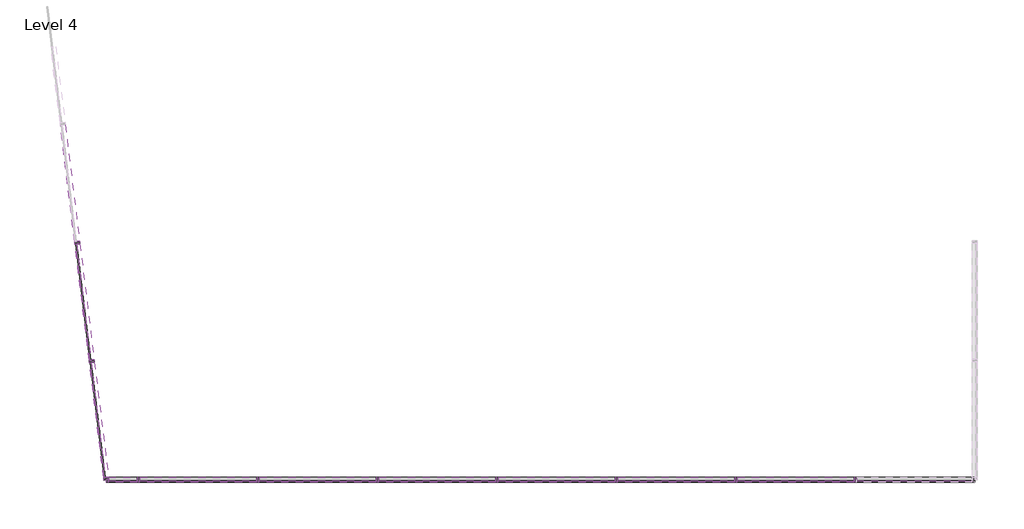
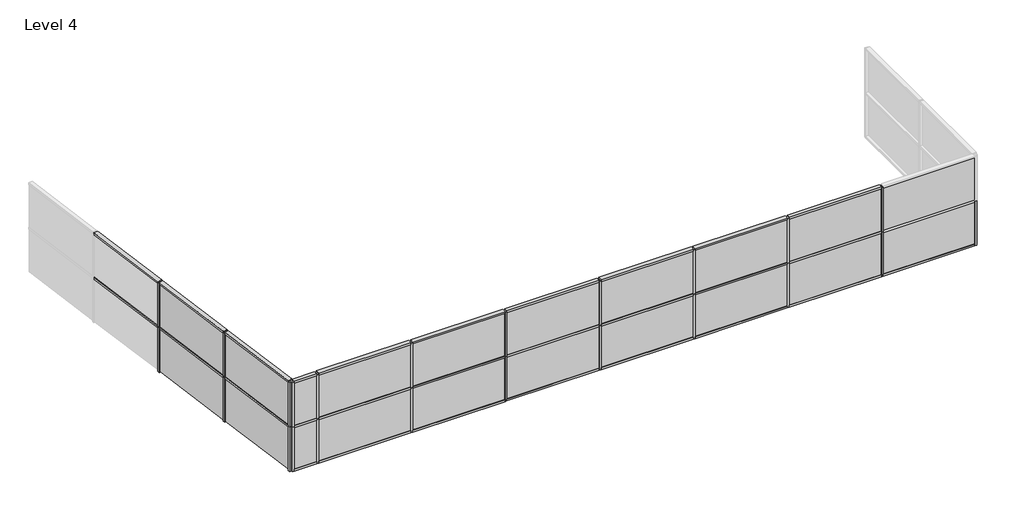
# One storey, part 1 of 2: 51 members, 20 plates.
"""IFC4 building model written with IfcOpenShell, lengths in millimetres."""

from ifc_helpers import new_model, si_unit, origin, place, context, project, spatial, transform, mapped, element, save
from components import member_71c27fd2, member_19d0a4ec, member_8cef0660, member_db480205, member_82905deb, member_4491d118, member_695b83e4, member_0c11e56c, system_panel_glazed_37f15d2e, system_panel_glazed_3620f98e, system_panel_glazed_e46d4b42, system_panel_glazed_2a6c68b7, system_panel_glazed_07b088f8, system_panel_glazed_9d0e0944

model = new_model("IFC4")

# Units and contexts
model_context = context("Model", 3, world=origin())
ifc_project = project(units=[si_unit("LENGTHUNIT", "METRE", prefix="MILLI")], contexts=[model_context])

# Site, building, storey
site = spatial("IfcSite", under=ifc_project)
building = spatial("IfcBuilding", under=site)
storey = spatial("IfcBuildingStorey", under=building, Name="Level 4", Elevation=9144.0)

# Members
placement = place(None, origin())
member_shape = member_71c27fd2(model_context)
element("IfcMember", 1, ObjectType="Rectangular Mullion : 2.5\" x 5\" rectangular", at=placement, inside=storey, context=model_context, shape_type="MappedRepresentation", body=[
    mapped(member_shape, transform((10886.265636, -6979.1363705, 9144.0), x_axis=(0.0, 0.0, -1.0), y_axis=(0.0, -1.0, 0.0), z_axis=(-1.0, 0.0, 0.0))),
])
member_2_shape = member_19d0a4ec(model_context)
element("IfcMember", 2, ObjectType="Rectangular Mullion : 2.5\" x 5\" rectangular", at=placement, inside=storey, context=model_context, shape_type="MappedRepresentation", body=[
    mapped(member_2_shape, transform((-8260.4765148, -6916.1096898, 10668.0), x_axis=(0.0, 0.0, 1.0), y_axis=(-0.9925461516413222, -0.12186934340514594, 0.0), z_axis=(0.12186934340514592, -0.9925461516413221, 0.0))),
])
element("IfcMember", 3, ObjectType="Rectangular Mullion : 2.5\" x 5\" rectangular", at=placement, inside=storey, context=model_context, shape_type="MappedRepresentation", body=[
    mapped(member_2_shape, transform((-8260.4765148, -6916.1096898, 12192.0), x_axis=(0.0, 0.0, 1.0), y_axis=(-0.9925461516413222, -0.1218693434051461, 0.0), z_axis=(0.1218693434051461, -0.9925461516413222, 0.0))),
])
member_3_shape = member_8cef0660(model_context)
element("IfcMember", 4, ObjectType="Rectangular Mullion : 2.5\" x 5\" rectangular", at=placement, inside=storey, context=model_context, shape_type="MappedRepresentation", body=[
    mapped(member_3_shape, transform((10822.765636, -6979.1363705, 10668.0), x_axis=(0.0, 0.0, 1.0), y_axis=(0.0, -1.0, 0.0), z_axis=(1.0, 0.0, 0.0))),
])
element("IfcMember", 5, ObjectType="Rectangular Mullion : 2.5\" x 5\" rectangular", at=placement, inside=storey, context=model_context, shape_type="MappedRepresentation", body=[
    mapped(member_3_shape, transform((7774.765636, -6979.1363705, 10668.0), x_axis=(0.0, 0.0, 1.0), y_axis=(0.0, -1.0, 0.0), z_axis=(1.0, 0.0, 0.0))),
])
element("IfcMember", 6, ObjectType="Rectangular Mullion : 2.5\" x 5\" rectangular", at=placement, inside=storey, context=model_context, shape_type="MappedRepresentation", body=[
    mapped(member_3_shape, transform((4726.765636, -6979.1363705, 10668.0), x_axis=(0.0, 0.0, 1.0), y_axis=(0.0, -1.0, 0.0), z_axis=(1.0, 0.0, 0.0))),
])
element("IfcMember", 7, ObjectType="Rectangular Mullion : 2.5\" x 5\" rectangular", at=placement, inside=storey, context=model_context, shape_type="MappedRepresentation", body=[
    mapped(member_3_shape, transform((1678.765636, -6979.1363705, 10668.0), x_axis=(0.0, 0.0, 1.0), y_axis=(0.0, -1.0, 0.0), z_axis=(1.0, 0.0, 0.0))),
])
element("IfcMember", 8, ObjectType="Rectangular Mullion : 2.5\" x 5\" rectangular", at=placement, inside=storey, context=model_context, shape_type="MappedRepresentation", body=[
    mapped(member_3_shape, transform((-1369.234364, -6979.1363705, 10668.0), x_axis=(0.0, 0.0, 1.0), y_axis=(0.0, -1.0, 0.0), z_axis=(1.0, 0.0, 0.0))),
])
element("IfcMember", 9, ObjectType="Rectangular Mullion : 2.5\" x 5\" rectangular", at=placement, inside=storey, context=model_context, shape_type="MappedRepresentation", body=[
    mapped(member_3_shape, transform((-4417.234364, -6979.1363705, 10668.0), x_axis=(0.0, 0.0, 1.0), y_axis=(0.0, -1.0, 0.0), z_axis=(1.0, 0.0, 0.0))),
])
element("IfcMember", 10, ObjectType="Rectangular Mullion : 2.5\" x 5\" rectangular", at=placement, inside=storey, context=model_context, shape_type="MappedRepresentation", body=[
    mapped(member_3_shape, transform((10822.765636, -6979.1363705, 12192.0), x_axis=(0.0, 0.0, 1.0), y_axis=(0.0, -1.0, 0.0), z_axis=(1.0, 0.0, 0.0))),
])
element("IfcMember", 11, ObjectType="Rectangular Mullion : 2.5\" x 5\" rectangular", at=placement, inside=storey, context=model_context, shape_type="MappedRepresentation", body=[
    mapped(member_3_shape, transform((7774.765636, -6979.1363705, 12192.0), x_axis=(0.0, 0.0, 1.0), y_axis=(0.0, -1.0, 0.0), z_axis=(1.0, 0.0, 0.0))),
])
element("IfcMember", 12, ObjectType="Rectangular Mullion : 2.5\" x 5\" rectangular", at=placement, inside=storey, context=model_context, shape_type="MappedRepresentation", body=[
    mapped(member_3_shape, transform((4726.765636, -6979.1363705, 12192.0), x_axis=(0.0, 0.0, 1.0), y_axis=(0.0, -1.0, 0.0), z_axis=(1.0, 0.0, 0.0))),
])
element("IfcMember", 13, ObjectType="Rectangular Mullion : 2.5\" x 5\" rectangular", at=placement, inside=storey, context=model_context, shape_type="MappedRepresentation", body=[
    mapped(member_3_shape, transform((1678.765636, -6979.1363705, 12192.0), x_axis=(0.0, 0.0, 1.0), y_axis=(0.0, -1.0, 0.0), z_axis=(1.0, 0.0, 0.0))),
])
element("IfcMember", 14, ObjectType="Rectangular Mullion : 2.5\" x 5\" rectangular", at=placement, inside=storey, context=model_context, shape_type="MappedRepresentation", body=[
    mapped(member_3_shape, transform((-1369.234364, -6979.1363705, 12192.0), x_axis=(0.0, 0.0, 1.0), y_axis=(0.0, -1.0, 0.0), z_axis=(1.0, 0.0, 0.0))),
])
element("IfcMember", 15, ObjectType="Rectangular Mullion : 2.5\" x 5\" rectangular", at=placement, inside=storey, context=model_context, shape_type="MappedRepresentation", body=[
    mapped(member_3_shape, transform((-4417.234364, -6979.1363705, 12192.0), x_axis=(0.0, 0.0, 1.0), y_axis=(0.0, -1.0, 0.0), z_axis=(1.0, 0.0, 0.0))),
])
element("IfcMember", 16, ObjectType="Rectangular Mullion : 2.5\" x 5\" rectangular", at=placement, inside=storey, context=model_context, shape_type="MappedRepresentation", body=[
    mapped(member_3_shape, transform((-8628.0649219, -3922.3423596, 10668.0), x_axis=(0.0, 0.0, 1.0), y_axis=(-0.9925461516413222, -0.12186934340514595, 0.0), z_axis=(0.12186934340514595, -0.9925461516413222, 0.0))),
])
element("IfcMember", 17, ObjectType="Rectangular Mullion : 2.5\" x 5\" rectangular", at=placement, inside=storey, context=model_context, shape_type="MappedRepresentation", body=[
    mapped(member_3_shape, transform((-8999.5226806, -897.0616894, 10668.0), x_axis=(0.0, 0.0, 1.0), y_axis=(-0.9925461516413222, -0.12186934340514602, 0.0), z_axis=(0.12186934340514602, -0.9925461516413222, 0.0))),
])
element("IfcMember", 18, ObjectType="Rectangular Mullion : 2.5\" x 5\" rectangular", at=placement, inside=storey, context=model_context, shape_type="MappedRepresentation", body=[
    mapped(member_3_shape, transform((-8628.0649219, -3922.3423596, 12192.0), x_axis=(0.0, 0.0, 1.0), y_axis=(-0.9925461516413222, -0.12186934340514595, 0.0), z_axis=(0.12186934340514595, -0.9925461516413222, 0.0))),
])
element("IfcMember", 19, ObjectType="Rectangular Mullion : 2.5\" x 5\" rectangular", at=placement, inside=storey, context=model_context, shape_type="MappedRepresentation", body=[
    mapped(member_3_shape, transform((-8999.5226806, -897.0616894, 12192.0), x_axis=(0.0, 0.0, 1.0), y_axis=(-0.9925461516413222, -0.12186934340514566, 0.0), z_axis=(0.12186934340514566, -0.9925461516413222, 0.0))),
])
member_4_shape = member_db480205(model_context)
element("IfcMember", 20, ObjectType="Rectangular Mullion : 2.5\" x 5\" rectangular", at=placement, inside=storey, context=model_context, shape_type="MappedRepresentation", body=[
    mapped(member_4_shape, transform((7838.265636, -6979.1363705, 9144.0), x_axis=(0.0, 0.0, -1.0), y_axis=(0.0, -1.0, 0.0), z_axis=(-1.0, 0.0, 0.0))),
])
element("IfcMember", 21, ObjectType="Rectangular Mullion : 2.5\" x 5\" rectangular", at=placement, inside=storey, context=model_context, shape_type="MappedRepresentation", body=[
    mapped(member_4_shape, transform((4790.265636, -6979.1363705, 9144.0), x_axis=(0.0, 0.0, -1.0), y_axis=(0.0, -1.0, 0.0), z_axis=(-1.0, 0.0, 0.0))),
])
element("IfcMember", 22, ObjectType="Rectangular Mullion : 2.5\" x 5\" rectangular", at=placement, inside=storey, context=model_context, shape_type="MappedRepresentation", body=[
    mapped(member_4_shape, transform((1742.265636, -6979.1363705, 9144.0), x_axis=(0.0, 0.0, -1.0), y_axis=(0.0, -1.0, 0.0), z_axis=(-1.0, 0.0, 0.0))),
])
element("IfcMember", 23, ObjectType="Rectangular Mullion : 2.5\" x 5\" rectangular", at=placement, inside=storey, context=model_context, shape_type="MappedRepresentation", body=[
    mapped(member_4_shape, transform((-1305.734364, -6979.1363705, 9144.0), x_axis=(0.0, 0.0, -1.0), y_axis=(0.0, -1.0, 0.0), z_axis=(-1.0, 0.0, 0.0))),
])
element("IfcMember", 24, ObjectType="Rectangular Mullion : 2.5\" x 5\" rectangular", at=placement, inside=storey, context=model_context, shape_type="MappedRepresentation", body=[
    mapped(member_4_shape, transform((-4353.734364, -6979.1363705, 9144.0), x_axis=(0.0, 0.0, -1.0), y_axis=(0.0, -1.0, 0.0), z_axis=(-1.0, 0.0, 0.0))),
])
element("IfcMember", 25, ObjectType="Rectangular Mullion : 2.5\" x 5\" rectangular", at=placement, inside=storey, context=model_context, shape_type="MappedRepresentation", body=[
    mapped(member_4_shape, transform((-7401.734364, -6979.1363705, 9144.0), x_axis=(0.0, 0.0, -1.0), y_axis=(0.0, -1.0, 0.0), z_axis=(-1.0, 0.0, 0.0))),
])
member_5_shape = member_82905deb(model_context)
element("IfcMember", 26, ObjectType="Rectangular Mullion : 2.5\" x 5\" rectangular", at=placement, inside=storey, context=model_context, shape_type="MappedRepresentation", body=[
    mapped(member_5_shape, transform((10854.515636, -6979.1363705, 10668.0), x_axis=(-1.0, 0.0, 0.0), y_axis=(0.0, -1.0, 0.0), z_axis=(0.0, 0.0, 1.0))),
])
element("IfcMember", 27, ObjectType="Rectangular Mullion : 2.5\" x 5\" rectangular", at=placement, inside=storey, context=model_context, shape_type="MappedRepresentation", body=[
    mapped(member_5_shape, transform((7806.515636, -6979.1363705, 10668.0), x_axis=(-1.0, 0.0, 0.0), y_axis=(0.0, -1.0, 0.0), z_axis=(0.0, 0.0, 1.0))),
])
element("IfcMember", 28, ObjectType="Rectangular Mullion : 2.5\" x 5\" rectangular", at=placement, inside=storey, context=model_context, shape_type="MappedRepresentation", body=[
    mapped(member_5_shape, transform((4758.515636, -6979.1363705, 10668.0), x_axis=(-1.0, 0.0, 0.0), y_axis=(0.0, -1.0, 0.0), z_axis=(0.0, 0.0, 1.0))),
])
element("IfcMember", 29, ObjectType="Rectangular Mullion : 2.5\" x 5\" rectangular", at=placement, inside=storey, context=model_context, shape_type="MappedRepresentation", body=[
    mapped(member_5_shape, transform((1710.515636, -6979.1363705, 10668.0), x_axis=(-1.0, 0.0, 0.0), y_axis=(0.0, -1.0, 0.0), z_axis=(0.0, 0.0, 1.0))),
])
element("IfcMember", 30, ObjectType="Rectangular Mullion : 2.5\" x 5\" rectangular", at=placement, inside=storey, context=model_context, shape_type="MappedRepresentation", body=[
    mapped(member_5_shape, transform((-1337.484364, -6979.1363705, 10668.0), x_axis=(-1.0, 0.0, 0.0), y_axis=(0.0, -1.0, 0.0), z_axis=(0.0, 0.0, 1.0))),
])
element("IfcMember", 31, ObjectType="Rectangular Mullion : 2.5\" x 5\" rectangular", at=placement, inside=storey, context=model_context, shape_type="MappedRepresentation", body=[
    mapped(member_5_shape, transform((-4385.484364, -6979.1363705, 10668.0), x_axis=(-1.0, 0.0, 0.0), y_axis=(0.0, -1.0, 0.0), z_axis=(0.0, 0.0, 1.0))),
])
element("IfcMember", 32, ObjectType="Rectangular Mullion : 2.5\" x 5\" rectangular", at=placement, inside=storey, context=model_context, shape_type="MappedRepresentation", body=[
    mapped(member_5_shape, transform((-7433.484364, -6979.1363705, 10668.0), x_axis=(-1.0, 0.0, 0.0), y_axis=(0.0, -1.0, 0.0), z_axis=(0.0, 0.0, 1.0))),
])
element("IfcMember", 33, ObjectType="Rectangular Mullion : 2.5\" x 5\" rectangular", at=placement, inside=storey, context=model_context, shape_type="MappedRepresentation", body=[
    mapped(member_5_shape, transform((10854.515636, -6979.1363705, 12192.0), x_axis=(-1.0, 0.0, 0.0), y_axis=(0.0, -1.0, 0.0), z_axis=(0.0, 0.0, 1.0))),
])
element("IfcMember", 34, ObjectType="Rectangular Mullion : 2.5\" x 5\" rectangular", at=placement, inside=storey, context=model_context, shape_type="MappedRepresentation", body=[
    mapped(member_5_shape, transform((7806.515636, -6979.1363705, 12192.0), x_axis=(-1.0, 0.0, 0.0), y_axis=(0.0, -1.0, 0.0), z_axis=(0.0, 0.0, 1.0))),
])
element("IfcMember", 35, ObjectType="Rectangular Mullion : 2.5\" x 5\" rectangular", at=placement, inside=storey, context=model_context, shape_type="MappedRepresentation", body=[
    mapped(member_5_shape, transform((4758.515636, -6979.1363705, 12192.0), x_axis=(-1.0, 0.0, 0.0), y_axis=(0.0, -1.0, 0.0), z_axis=(0.0, 0.0, 1.0))),
])
element("IfcMember", 36, ObjectType="Rectangular Mullion : 2.5\" x 5\" rectangular", at=placement, inside=storey, context=model_context, shape_type="MappedRepresentation", body=[
    mapped(member_5_shape, transform((1710.515636, -6979.1363705, 12192.0), x_axis=(-1.0, 0.0, 0.0), y_axis=(0.0, -1.0, 0.0), z_axis=(0.0, 0.0, 1.0))),
])
element("IfcMember", 37, ObjectType="Rectangular Mullion : 2.5\" x 5\" rectangular", at=placement, inside=storey, context=model_context, shape_type="MappedRepresentation", body=[
    mapped(member_5_shape, transform((-1337.484364, -6979.1363705, 12192.0), x_axis=(-1.0, 0.0, 0.0), y_axis=(0.0, -1.0, 0.0), z_axis=(0.0, 0.0, 1.0))),
])
element("IfcMember", 38, ObjectType="Rectangular Mullion : 2.5\" x 5\" rectangular", at=placement, inside=storey, context=model_context, shape_type="MappedRepresentation", body=[
    mapped(member_5_shape, transform((-4385.484364, -6979.1363705, 12192.0), x_axis=(-1.0, 0.0, 0.0), y_axis=(0.0, -1.0, 0.0), z_axis=(0.0, 0.0, 1.0))),
])
element("IfcMember", 39, ObjectType="Rectangular Mullion : 2.5\" x 5\" rectangular", at=placement, inside=storey, context=model_context, shape_type="MappedRepresentation", body=[
    mapped(member_5_shape, transform((-7433.484364, -6979.1363705, 12192.0), x_axis=(-1.0, 0.0, 0.0), y_axis=(0.0, -1.0, 0.0), z_axis=(0.0, 0.0, 1.0))),
])
element("IfcMember", 40, ObjectType="Rectangular Mullion : 2.5\" x 5\" rectangular", at=placement, inside=storey, context=model_context, shape_type="MappedRepresentation", body=[
    mapped(member_5_shape, transform((-8624.1955702, -3953.8557, 10668.0), x_axis=(-0.1218693434051459, 0.9925461516413222, 0.0), y_axis=(-0.9925461516413222, -0.1218693434051459, 0.0), z_axis=(0.0, 0.0, 1.0))),
])
element("IfcMember", 41, ObjectType="Rectangular Mullion : 2.5\" x 5\" rectangular", at=placement, inside=storey, context=model_context, shape_type="MappedRepresentation", body=[
    mapped(member_5_shape, transform((-8624.1955702, -3953.8557, 12192.0), x_axis=(-0.1218693434051459, 0.9925461516413222, 0.0), y_axis=(-0.9925461516413222, -0.1218693434051459, 0.0), z_axis=(0.0, 0.0, 1.0))),
])
element("IfcMember", 42, ObjectType="Rectangular Mullion : 2.5\" x 5\" rectangular", at=placement, inside=storey, context=model_context, shape_type="MappedRepresentation", body=[
    mapped(member_5_shape, transform((-8995.6533289, -928.5750297, 10668.0), x_axis=(-0.1218693434051459, 0.9925461516413222, 0.0), y_axis=(-0.9925461516413222, -0.1218693434051459, 0.0), z_axis=(0.0, 0.0, 1.0))),
])
element("IfcMember", 43, ObjectType="Rectangular Mullion : 2.5\" x 5\" rectangular", at=placement, inside=storey, context=model_context, shape_type="MappedRepresentation", body=[
    mapped(member_5_shape, transform((-8995.6533289, -928.5750297, 12192.0), x_axis=(-0.1218693434051459, 0.9925461516413222, 0.0), y_axis=(-0.9925461516413222, -0.1218693434051459, 0.0), z_axis=(0.0, 0.0, 1.0))),
])
member_6_shape = member_4491d118(model_context)
element("IfcMember", 44, ObjectType="Rectangular Mullion : 2.5\" x 5\" rectangular", at=placement, inside=storey, context=model_context, shape_type="MappedRepresentation", body=[
    mapped(member_6_shape, transform((13902.5156363, -6979.1363705, 9144.0), x_axis=(1.0, 0.0, 0.0), y_axis=(0.0, -1.0, 0.0), z_axis=(0.0, 0.0, -1.0))),
])
element("IfcMember", 45, ObjectType="Rectangular Mullion : 2.5\" x 5\" rectangular", at=placement, inside=storey, context=model_context, shape_type="MappedRepresentation", body=[
    mapped(member_6_shape, transform((-8252.7378115, -6979.1363705, 9144.0), x_axis=(0.1218693434051459, -0.9925461516413222, 0.0), y_axis=(-0.9925461516413222, -0.1218693434051459, 0.0), z_axis=(0.0, 0.0, -1.0))),
])
element("IfcMember", 46, ObjectType="Rectangular Mullion : 2.5\" x 5\" rectangular", at=placement, inside=storey, context=model_context, shape_type="MappedRepresentation", body=[
    mapped(member_6_shape, transform((-8252.7378115, -6979.1363705, 10668.0), x_axis=(0.1218693434051459, -0.9925461516413222, 0.0), y_axis=(-0.9925461516413222, -0.1218693434051459, 0.0), z_axis=(0.0, 0.0, -1.0))),
])
element("IfcMember", 47, ObjectType="Rectangular Mullion : 2.5\" x 5\" rectangular", at=placement, inside=storey, context=model_context, shape_type="MappedRepresentation", body=[
    mapped(member_6_shape, transform((-8252.7378115, -6979.1363705, 10668.0), x_axis=(-1.0, 0.0, 0.0), y_axis=(0.0, -1.0, 0.0), z_axis=(0.0, 0.0, 1.0))),
])
element("IfcMember", 48, ObjectType="Rectangular Mullion : 2.5\" x 5\" rectangular", at=placement, inside=storey, context=model_context, shape_type="MappedRepresentation", body=[
    mapped(member_6_shape, transform((-8252.7378115, -6979.1363705, 12192.0), x_axis=(-1.0, 0.0, 0.0), y_axis=(0.0, -1.0, 0.0), z_axis=(0.0, 0.0, 1.0))),
])
member_7_shape = member_695b83e4(model_context)
element("IfcMember", 49, ObjectType="Rectangular Mullion : 2.5\" x 5\" rectangular", at=placement, inside=storey, context=model_context, shape_type="MappedRepresentation", body=[
    mapped(member_7_shape, transform((-8189.2378115, -6979.1363705, 9144.0), x_axis=(0.0, 0.0, -1.0), y_axis=(0.0, -1.0, 0.0), z_axis=(-1.0, 0.0, 0.0))),
])
member_8_shape = member_0c11e56c(model_context)
element("IfcMember", 50, ObjectType="Rectangular Mullion : 2.5\" x 5\" rectangular", at=placement, inside=storey, context=model_context, shape_type="MappedRepresentation", body=[
    mapped(member_8_shape, transform((-7465.234364, -6979.1363705, 10668.0), x_axis=(0.0, 0.0, 1.0), y_axis=(0.0, -1.0, 0.0), z_axis=(1.0, 0.0, 0.0))),
])
element("IfcMember", 51, ObjectType="Rectangular Mullion : 2.5\" x 5\" rectangular", at=placement, inside=storey, context=model_context, shape_type="MappedRepresentation", body=[
    mapped(member_8_shape, transform((-7465.234364, -6979.1363705, 12192.0), x_axis=(0.0, 0.0, 1.0), y_axis=(0.0, -1.0, 0.0), z_axis=(1.0, 0.0, 0.0))),
])

# Plates
system_panel_glazed_shape = system_panel_glazed_37f15d2e(model_context)
element("IfcPlate", 52, ObjectType="System Panel : Glazed", at=placement, inside=storey, context=model_context, shape_type="MappedRepresentation", body=[
    mapped(system_panel_glazed_shape, transform((12362.6406361, -6979.1363705, 9207.5), x_axis=(-1.0, 0.0, 0.0), y_axis=(0.0, -1.0, 0.0), z_axis=(0.0, 0.0, 1.0))),
])
system_panel_glazed_2_shape = system_panel_glazed_3620f98e(model_context)
element("IfcPlate", 53, ObjectType="System Panel : Glazed", at=placement, inside=storey, context=model_context, shape_type="MappedRepresentation", body=[
    mapped(system_panel_glazed_2_shape, transform((9330.515636, -6979.1363705, 9207.5), x_axis=(-1.0, 0.0, 0.0), y_axis=(0.0, -1.0, 0.0), z_axis=(0.0, 0.0, 1.0))),
])
element("IfcPlate", 54, ObjectType="System Panel : Glazed", at=placement, inside=storey, context=model_context, shape_type="MappedRepresentation", body=[
    mapped(system_panel_glazed_2_shape, transform((6282.515636, -6979.1363705, 9207.5), x_axis=(-1.0, 0.0, 0.0), y_axis=(0.0, -1.0, 0.0), z_axis=(0.0, 0.0, 1.0))),
])
element("IfcPlate", 55, ObjectType="System Panel : Glazed", at=placement, inside=storey, context=model_context, shape_type="MappedRepresentation", body=[
    mapped(system_panel_glazed_2_shape, transform((3234.515636, -6979.1363705, 9207.5), x_axis=(-1.0, 0.0, 0.0), y_axis=(0.0, -1.0, 0.0), z_axis=(0.0, 0.0, 1.0))),
])
element("IfcPlate", 56, ObjectType="System Panel : Glazed", at=placement, inside=storey, context=model_context, shape_type="MappedRepresentation", body=[
    mapped(system_panel_glazed_2_shape, transform((186.515636, -6979.1363705, 9207.5), x_axis=(-1.0, 0.0, 0.0), y_axis=(0.0, -1.0, 0.0), z_axis=(0.0, 0.0, 1.0))),
])
element("IfcPlate", 57, ObjectType="System Panel : Glazed", at=placement, inside=storey, context=model_context, shape_type="MappedRepresentation", body=[
    mapped(system_panel_glazed_2_shape, transform((-2861.484364, -6979.1363705, 9207.5), x_axis=(-1.0, 0.0, 0.0), y_axis=(0.0, -1.0, 0.0), z_axis=(0.0, 0.0, 1.0))),
])
element("IfcPlate", 58, ObjectType="System Panel : Glazed", at=placement, inside=storey, context=model_context, shape_type="MappedRepresentation", body=[
    mapped(system_panel_glazed_2_shape, transform((-5909.484364, -6979.1363705, 9207.5), x_axis=(-1.0, 0.0, 0.0), y_axis=(0.0, -1.0, 0.0), z_axis=(0.0, 0.0, 1.0))),
])
system_panel_glazed_3_shape = system_panel_glazed_e46d4b42(model_context)
element("IfcPlate", 59, ObjectType="System Panel : Glazed", at=placement, inside=storey, context=model_context, shape_type="MappedRepresentation", body=[
    mapped(system_panel_glazed_3_shape, transform((-8440.4013667, -5450.739365, 9175.75), x_axis=(-0.1218693434051459, 0.9925461516413222, 0.0), y_axis=(-0.9925461516413222, -0.1218693434051459, 0.0), z_axis=(0.0, 0.0, 1.0))),
])
element("IfcPlate", 60, ObjectType="System Panel : Glazed", at=placement, inside=storey, context=model_context, shape_type="MappedRepresentation", body=[
    mapped(system_panel_glazed_3_shape, transform((-8440.4013667, -5450.739365, 10699.75), x_axis=(-0.1218693434051459, 0.9925461516413222, 0.0), y_axis=(-0.9925461516413222, -0.1218693434051459, 0.0), z_axis=(0.0, 0.0, 1.0))),
])
element("IfcPlate", 61, ObjectType="System Panel : Glazed", at=placement, inside=storey, context=model_context, shape_type="MappedRepresentation", body=[
    mapped(system_panel_glazed_3_shape, transform((12362.6406361, -6979.1363705, 10699.75), x_axis=(-1.0, 0.0, 0.0), y_axis=(0.0, -1.0, 0.0), z_axis=(0.0, 0.0, 1.0))),
])
system_panel_glazed_4_shape = system_panel_glazed_2a6c68b7(model_context)
element("IfcPlate", 62, ObjectType="System Panel : Glazed", at=placement, inside=storey, context=model_context, shape_type="MappedRepresentation", body=[
    mapped(system_panel_glazed_4_shape, transform((-8809.9244496, -2441.2153649, 9175.75), x_axis=(-0.1218693434051459, 0.9925461516413222, 0.0), y_axis=(-0.9925461516413222, -0.1218693434051459, 0.0), z_axis=(0.0, 0.0, 1.0))),
])
element("IfcPlate", 63, ObjectType="System Panel : Glazed", at=placement, inside=storey, context=model_context, shape_type="MappedRepresentation", body=[
    mapped(system_panel_glazed_4_shape, transform((-8809.9244496, -2441.2153649, 10699.75), x_axis=(-0.1218693434051459, 0.9925461516413222, 0.0), y_axis=(-0.9925461516413222, -0.1218693434051459, 0.0), z_axis=(0.0, 0.0, 1.0))),
])
element("IfcPlate", 64, ObjectType="System Panel : Glazed", at=placement, inside=storey, context=model_context, shape_type="MappedRepresentation", body=[
    mapped(system_panel_glazed_4_shape, transform((9330.515636, -6979.1363705, 10699.75), x_axis=(-1.0, 0.0, 0.0), y_axis=(0.0, -1.0, 0.0), z_axis=(0.0, 0.0, 1.0))),
])
element("IfcPlate", 65, ObjectType="System Panel : Glazed", at=placement, inside=storey, context=model_context, shape_type="MappedRepresentation", body=[
    mapped(system_panel_glazed_4_shape, transform((6282.515636, -6979.1363705, 10699.75), x_axis=(-1.0, 0.0, 0.0), y_axis=(0.0, -1.0, 0.0), z_axis=(0.0, 0.0, 1.0))),
])
element("IfcPlate", 66, ObjectType="System Panel : Glazed", at=placement, inside=storey, context=model_context, shape_type="MappedRepresentation", body=[
    mapped(system_panel_glazed_4_shape, transform((3234.515636, -6979.1363705, 10699.75), x_axis=(-1.0, 0.0, 0.0), y_axis=(0.0, -1.0, 0.0), z_axis=(0.0, 0.0, 1.0))),
])
element("IfcPlate", 67, ObjectType="System Panel : Glazed", at=placement, inside=storey, context=model_context, shape_type="MappedRepresentation", body=[
    mapped(system_panel_glazed_4_shape, transform((186.515636, -6979.1363705, 10699.75), x_axis=(-1.0, 0.0, 0.0), y_axis=(0.0, -1.0, 0.0), z_axis=(0.0, 0.0, 1.0))),
])
element("IfcPlate", 68, ObjectType="System Panel : Glazed", at=placement, inside=storey, context=model_context, shape_type="MappedRepresentation", body=[
    mapped(system_panel_glazed_4_shape, transform((-2861.484364, -6979.1363705, 10699.75), x_axis=(-1.0, 0.0, 0.0), y_axis=(0.0, -1.0, 0.0), z_axis=(0.0, 0.0, 1.0))),
])
element("IfcPlate", 69, ObjectType="System Panel : Glazed", at=placement, inside=storey, context=model_context, shape_type="MappedRepresentation", body=[
    mapped(system_panel_glazed_4_shape, transform((-5909.484364, -6979.1363705, 10699.75), x_axis=(-1.0, 0.0, 0.0), y_axis=(0.0, -1.0, 0.0), z_axis=(0.0, 0.0, 1.0))),
])
system_panel_glazed_5_shape = system_panel_glazed_07b088f8(model_context)
element("IfcPlate", 70, ObjectType="System Panel : Glazed", at=placement, inside=storey, context=model_context, shape_type="MappedRepresentation", body=[
    mapped(system_panel_glazed_5_shape, transform((-7827.2360878, -6979.1363705, 9207.5), x_axis=(-1.0, 0.0, 0.0), y_axis=(0.0, -1.0, 0.0), z_axis=(0.0, 0.0, 1.0))),
])
system_panel_glazed_6_shape = system_panel_glazed_9d0e0944(model_context)
element("IfcPlate", 71, ObjectType="System Panel : Glazed", at=placement, inside=storey, context=model_context, shape_type="MappedRepresentation", body=[
    mapped(system_panel_glazed_6_shape, transform((-7827.2360878, -6979.1363705, 10699.75), x_axis=(-1.0, 0.0, 0.0), y_axis=(0.0, -1.0, 0.0), z_axis=(0.0, 0.0, 1.0))),
])

save(model, "model.ifc")

# Revit data of these elements
# Type "Rectangular Mullion : 2.5\" x 5\" rectangular"
#   built-in parameter 1007304 = 0.416667 (stored number, unit not read)
#   built-in parameter 1007301 = 0.104167 (stored number, unit not read)
#   built-in parameter 1007300 = 0.104167 (stored number, unit not read)
# Type "System Panel : Glazed"
#   Construction Type Id = "GSP4R"
#   Analytic Construction = "1/8 in Pilkington single glazing"
#   Visual Light Transmittance = 0.9
#   Solar Heat Gain Coefficient = 0.86
#   Heat Transfer Coefficient (U) = 1.18115 BTU/(h·ft²·°F)
#   Define Thermal Properties by = 1
# Elements 1, 2, 3, 4, 5, 6, 7, 8, 9, 10, 11, 12, 13, 14, 15, 16, 17, 18, 19, 20, 21, 22, 23, 24, 25, 26, 27, 28, 29, 30, 31, 32, 33, 34, 35, 36, 37, 38, 39, 40, 41, 42, 43, 44, 45, 46, 47, 48, 49, 50, 51 (IfcMember, "Rectangular Mullion : 2.5\" x 5\" rectangular")
#   Phase Created = New Construction
#   Materials on its faces: "Aluminum"
# Elements 52, 53, 54, 55, 56, 57, 58, 59, 60, 61, 62, 63, 64, 65, 66, 67, 68, 69, 70, 71 (IfcPlate, "System Panel : Glazed")
#   Phase Created = New Construction
#   Materials on its faces: "Glass"
# Materials
#   "Aluminum": class "Metal", colour RGB 247 247 247, transparency 0, Description = "Aluminum 6061", Cost = 0
#   "Glass": class "Glass", colour RGB 0 128 192, transparency 0.75, Description = "Soda Lime Glass", Cost = 0
